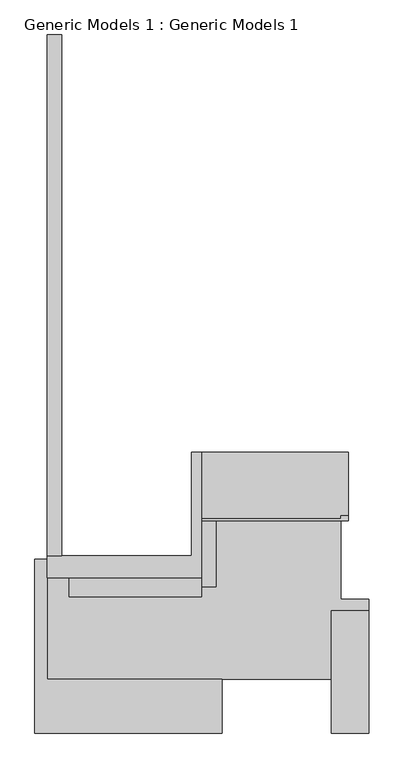
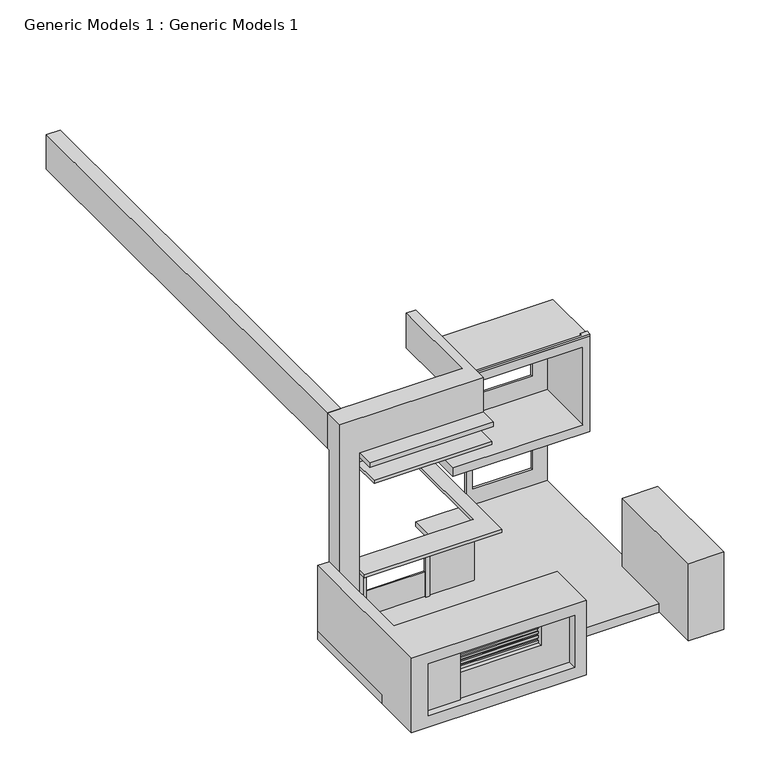
"""IFC4 building model written with IfcOpenShell, lengths in millimetres: proxy geometry, Generic Models 1 : Generic Models 1."""

from ifc_helpers import new_model, si_unit, frame, origin, place, context, project, spatial, polyline, outline, extrude, faceted_brep, source, transform, mapped, element, save


def generic_models_1_generic_models_1_aa7367fc(model_context):
    return source(origin(), model_context, "Body", "SolidModel", [
        extrude(outline(polyline([(-18721.6590927, -15995.5795999), (-19915.2161422, -15995.5795999), (-19915.2161422, -15919.3795999), (-18721.6590927, -15919.3795999), (-18721.6590927, -15995.5795999)])), frame((0.0, 0.0, 243.5207703), z_axis=(0.0, 0.0, 1.0), x_axis=(1.0, 0.0, 0.0)), (0.0, 0.0, 1.0), 1828.8),
        faceted_brep([(-20093.0161422, -14542.885934, 2459.7933128), (-20093.0161422, -10818.9867758, 2459.7933128), (-20474.0161422, -10818.9867758, 2459.7933128), (-20474.0161422, -16224.1795999, 2459.7933128), (-14644.7161422, -16224.1795999, 2459.7933128), (-14644.7161422, -14542.885934, 2459.7933128), (-20474.0161422, -14542.885934, 152.4), (-20474.0161422, -10818.9867758, 152.4), (-20093.0161422, -10818.9867758, 152.4), (-20093.0161422, -14542.885934, 152.4), (-20474.0161422, -14542.885934, -152.4), (-20474.0161422, -16224.1795999, -152.4), (-14644.7161422, -16224.1795999, -152.4), (-15038.4161422, -16224.1795999, 2072.3207703), (-15038.4161422, -16224.1795999, 243.5207703), (-19915.2161422, -16224.1795999, 243.5207703), (-19915.2161422, -16224.1795999, 2072.3207703), (-14644.7161422, -14542.885934, -152.4), (-19915.2161422, -15919.3795999, 2072.3207703), (-19915.2161422, -15919.3795999, 243.5207703), (-15038.4161422, -15919.3795999, 243.5207703), (-15038.4161422, -15919.3795999, 2072.3207703), (-15978.4590927, -15919.3795999, 2072.3207703), (-15978.4590927, -15919.3795999, 1157.9207703), (-18721.6590927, -15919.3795999, 1157.9207703), (-18721.6590927, -15919.3795999, 2072.3207703), (-18721.6590927, -15766.9795999, 2072.3207703), (-15978.4590927, -15766.9795999, 2072.3207703), (-18721.6590927, -15766.9795999, 1981.5649803), (-15978.4590927, -15766.9795999, 1981.5649803), (-18721.6590927, -15766.9795999, 1157.9207703), (-15978.4590927, -15766.9795999, 1157.9207703), (-15978.4590927, -15766.9795999, 1255.1713252), (-18721.6590927, -15766.9795999, 1255.1713252), (-18721.6590927, -15766.9795999, 1838.3053525), (-18721.6590927, -15766.9795999, 1778.0550652), (-15978.4590927, -15766.9795999, 1778.0550652), (-15978.4590927, -15766.9795999, 1838.3053525), (-18721.6590927, -15766.9795999, 1718.5907977), (-18721.6590927, -15766.9795999, 1668.7672478), (-15978.4590927, -15766.9795999, 1668.7672478), (-15978.4590927, -15766.9795999, 1718.5907977), (-18721.6590927, -15766.9795999, 1558.4809342), (-18721.6590927, -15766.9795999, 1493.486018), (-15978.4590927, -15766.9795999, 1493.486018), (-15978.4590927, -15766.9795999, 1558.4809342), (-18721.6590927, -15766.9795999, 1415.4921185), (-18721.6590927, -15766.9795999, 1328.8322303), (-15978.4590927, -15766.9795999, 1328.8322303), (-15978.4590927, -15766.9795999, 1415.4921185), (-15978.4590927, -15716.1795999, 1981.5649803), (-15978.4590927, -15716.1795999, 1838.3053525), (-15978.4590927, -15716.1795999, 1778.0550652), (-15978.4590927, -15716.1795999, 1718.5907977), (-15978.4590927, -15716.1795999, 1668.7672478), (-15978.4590927, -15716.1795999, 1558.4809342), (-15978.4590927, -15716.1795999, 1493.486018), (-15978.4590927, -15716.1795999, 1415.4921185), (-15978.4590927, -15716.1795999, 1328.8322303), (-15978.4590927, -15716.1795999, 1255.1713252), (-18721.6590927, -15716.1795999, 1255.1713252), (-18721.6590927, -15716.1795999, 1328.8322303), (-18721.6590927, -15716.1795999, 1415.4921185), (-18721.6590927, -15716.1795999, 1493.486018), (-18721.6590927, -15716.1795999, 1558.4809342), (-18721.6590927, -15716.1795999, 1668.7672478), (-18721.6590927, -15716.1795999, 1718.5907977), (-18721.6590927, -15716.1795999, 1778.0550652), (-18721.6590927, -15716.1795999, 1838.3053525), (-18721.6590927, -15716.1795999, 1981.5649803)], [[[0, 1, 2, 3, 4, 5]], [[6, 7, 8, 9]], [[1, 0, 9, 8]], [[2, 1, 8, 7]], [[7, 6, 10, 11, 3, 2]], [[12, 4, 3, 11], [13, 14, 15, 16]], [[17, 10, 6, 9, 0, 5]], [[4, 12, 17, 5]], [[12, 11, 10, 17]], [[18, 19, 20, 21, 22, 23, 24, 25]], [[21, 20, 14, 13]], [[20, 19, 15, 14]], [[19, 18, 16, 15]], [[21, 13, 16, 18, 25, 26, 27, 22]], [[27, 26, 28, 29]], [[30, 31, 32, 33]], [[34, 35, 36, 37]], [[38, 39, 40, 41]], [[42, 43, 44, 45]], [[46, 47, 48, 49]], [[31, 23, 22, 27, 29, 50, 51, 37, 36, 52, 53, 41, 40, 54, 55, 45, 44, 56, 57, 49, 48, 58, 59, 32]], [[31, 30, 24, 23]], [[24, 30, 33, 60, 61, 47, 46, 62, 63, 43, 42, 64, 65, 39, 38, 66, 67, 35, 34, 68, 69, 28, 26, 25]], [[50, 69, 68, 51]], [[52, 67, 66, 53]], [[54, 65, 64, 55]], [[56, 63, 62, 57]], [[58, 61, 60, 59]], [[51, 68, 34, 37]], [[69, 50, 29, 28]], [[53, 66, 38, 41]], [[67, 52, 36, 35]], [[55, 64, 42, 45]], [[65, 54, 40, 39]], [[57, 62, 46, 49]], [[63, 56, 44, 43]], [[59, 60, 33, 32]], [[61, 58, 48, 47]]]),
        extrude(outline(polyline([(-10072.7161422, -16224.1795999), (-11248.8984734, -16224.1795999), (-11248.8984734, -12419.1867758), (-10072.7161422, -12419.1867758), (-10072.7161422, -16224.1795999)])), frame((0.0, 0.0, -152.4), z_axis=(0.0, 0.0, 1.0), x_axis=(1.0, 0.0, 0.0)), (0.0, 0.0, 1.0), 2716.6580235),
        faceted_brep([(-19413.0681274, -10971.3867758, 2163.0020846), (-19413.0681274, -10971.3867758, 152.4), (-19038.9161422, -10971.3867758, 152.4), (-19038.9161422, -10971.3867758, 2163.0020846), (-19413.0681274, -10920.5867758, 2163.0020846), (-19038.9161422, -10920.5867758, 2163.0020846), (-19038.9161422, -10920.5867758, 152.4), (-19413.0681274, -10920.5867758, 152.4), (-18911.9161422, -10920.5867758, 2163.0020846), (-18911.9161422, -10920.5867758, 152.4), (-19038.9161422, -10818.9867758, 152.4), (-19038.9161422, -10818.9867758, 2163.0020846), (-18911.9161422, -10818.9867758, 2163.0020846), (-18911.9161422, -10818.9867758, 1025.0994511), (-16930.7161422, -10818.9867758, 1025.0994511), (-16930.7161422, -10818.9867758, 152.4), (-16930.7161422, -10869.7867758, 152.4), (-18911.9161422, -10869.7867758, 152.4), (-18911.9161422, -10869.7867758, 1025.0994511), (-16930.7161422, -10869.7867758, 1025.0994511)], [[[0, 1, 2, 3]], [[4, 5, 6, 7]], [[1, 0, 4, 7]], [[2, 1, 7, 6]], [[3, 2, 6, 5]], [[0, 3, 5, 4]], [[8, 5, 6, 9]], [[10, 11, 12, 13, 14, 15]], [[5, 8, 12, 11]], [[11, 10, 6, 5]], [[9, 6, 10, 15, 16, 17]], [[8, 9, 17, 18, 13, 12]], [[19, 18, 17, 16]], [[18, 19, 14, 13]], [[19, 16, 15, 14]]]),
        extrude(outline(polyline([(-15292.4161422, -10869.7867758), (-16802.5911072, -10869.7867758), (-16802.5911072, -10818.9867758), (-15292.4161422, -10818.9867758), (-15292.4161422, -10869.7867758)])), frame((0.0, 0.0, 152.4), z_axis=(0.0, 0.0, 1.0), x_axis=(1.0, 0.0, 0.0)), (0.0, 0.0, 1.0), 2010.6020846),
        extrude(outline(polyline([(-19219.0295013, -10869.7867758), (-19413.0681274, -10869.7867758), (-19413.0681274, -10818.9867758), (-19219.0295013, -10818.9867758), (-19219.0295013, -10869.7867758)])), frame((0.0, 0.0, 3352.8), z_axis=(0.0, 0.0, 1.0), x_axis=(1.0, 0.0, 0.0)), (0.0, 0.0, 1.0), 2310.6651167),
        extrude(outline(polyline([(-15292.4161422, -10869.7867758), (-19413.0681274, -10869.7867758), (-19413.0681274, -10818.9867758), (-15292.4161422, -10818.9867758), (-15292.4161422, -10869.7867758)])), frame((0.0, 0.0, 5663.4651167), z_axis=(0.0, 0.0, 1.0), x_axis=(1.0, 0.0, 0.0)), (0.0, 0.0, 1.0), 580.3392162),
        extrude(outline(polyline([(-16802.5911072, -10920.5867758), (-16930.7161422, -10920.5867758), (-16930.7161422, -10818.9867758), (-16802.5911072, -10818.9867758), (-16802.5911072, -10920.5867758)])), frame((0.0, 0.0, 152.4), z_axis=(0.0, 0.0, 1.0), x_axis=(1.0, 0.0, 0.0)), (0.0, 0.0, 1.0), 2010.6020846),
        extrude(outline(polyline([(2217.8846358, -10944.2876245), (3048.0, -10944.2876245), (3048.0, -13650.3561315), (152.4, -13650.3561315), (152.4, -10949.0161422), (2217.8846358, -10949.0161422), (2217.8846358, -10944.2876245)]), holes=[polyline([(2217.8846358, -11444.3161422), (714.2961729, -11444.3161422), (714.2961729, -13425.5161422), (2217.8846358, -13425.5161422), (2217.8846358, -11444.3161422)])]), frame((0.0, -7567.7867758, 0.0), z_axis=(0.0, 1.0, 0.0), x_axis=(0.0, 0.0, 1.0)), (0.0, 0.0, 1.0), 76.2),
        extrude(outline(polyline([(-19635.8161422, -10704.6867758), (-20093.0161422, -10704.6867758), (-20093.0161422, 5487.8132242), (-19635.8161422, 5487.8132242), (-19635.8161422, -10704.6867758)])), frame((0.0, 0.0, 6400.8), z_axis=(0.0, 0.0, 1.0), x_axis=(1.0, 0.0, 0.0)), (0.0, 0.0, 1.0), 1219.2),
        extrude(outline(polyline([(6096.0, -13658.1564563), (3352.8, -13658.1564563), (3352.8, -13425.5161422), (3355.4784757, -13425.5161422), (3355.4784757, -10949.0161422), (6096.0, -10949.0161422), (6096.0, -13658.1564563)]), holes=[polyline([(5431.5526731, -11457.0161422), (3998.6028627, -11457.0161422), (3998.6028627, -13425.5161422), (5431.5526731, -13425.5161422), (5431.5526731, -11457.0161422)])]), frame((0.0, -7567.7867758, 0.0), z_axis=(0.0, 1.0, 0.0), x_axis=(0.0, 0.0, 1.0)), (0.0, 0.0, 1.0), 76.2),
        extrude(outline(polyline([(-10720.4161422, -9625.1422165), (-15292.4161422, -9625.1422165), (-15292.4161422, -9563.1336072), (-10949.0161422, -9563.1336072), (-10949.0161422, -9466.2958238), (-10720.4161422, -9466.2958238), (-10720.4161422, -9625.1422165)])), frame((0.0, 0.0, 6400.8), z_axis=(0.0, 0.0, 1.0), x_axis=(1.0, 0.0, 0.0)), (0.0, 0.0, 1.0), 76.2),
        extrude(outline(polyline([(-19413.0681274, -11671.4830509), (-19413.0681274, -10818.9867758), (-15292.4161422, -10818.9867758), (-15292.4161422, -7516.9867758), (-14829.7614132, -7516.9867758), (-14829.7614132, -11671.4830509), (-19413.0681274, -11671.4830509)])), frame((0.0, 0.0, 2163.0020846), z_axis=(0.0, 0.0, 1.0), x_axis=(1.0, 0.0, 0.0)), (0.0, 0.0, 1.0), 101.6),
        extrude(outline(polyline([(-15292.4161422, -10818.9867758), (-15292.4161422, -11897.0390885), (-19216.7161422, -11897.0390885), (-19216.7161422, -10818.9867758), (-15292.4161422, -10818.9867758)])), frame((0.0, 0.0, 5554.6402073), z_axis=(0.0, 0.0, 1.0), x_axis=(1.0, 0.0, 0.0)), (0.0, 0.0, 1.0), 105.6615052),
        extrude(outline(polyline([(-15292.4161422, -11984.5426097), (-19413.0681274, -11984.5426097), (-19413.0681274, -10818.9867758), (-15292.4161422, -10818.9867758), (-15292.4161422, -11984.5426097)])), frame((0.0, 0.0, 6243.8043329), z_axis=(0.0, 0.0, 1.0), x_axis=(1.0, 0.0, 0.0)), (0.0, 0.0, 1.0), 156.9956671),
        faceted_brep([(-20093.0161422, -11395.0766858, 152.4), (-20093.0161422, -11395.0766858, 7620.0), (-20093.0161422, -10704.6867758, 7620.0), (-20093.0161422, -10704.6867758, 6400.8), (-20093.0161422, -10818.9867758, 6400.8), (-20093.0161422, -10818.9867758, 152.4), (-19413.0681274, -11395.0766858, 152.4), (-19413.0681274, -10818.9867758, 152.4), (-19413.0681274, -11395.0766858, 6400.8), (-19413.0681274, -10818.9867758, 6400.8), (-15597.2161422, -7491.5867758, 7620.0), (-15292.4161422, -7491.5867758, 7620.0), (-15292.4161422, -7491.5867758, 6400.8), (-15597.2161422, -7491.5867758, 6400.8), (-15597.2161422, -10704.6867758, 6400.8), (-15597.2161422, -10704.6867758, 7620.0), (-15292.4161422, -11395.0766858, 6400.8), (-15292.4161422, -11395.0766858, 7620.0)], [[[0, 1, 2, 3, 4, 5]], [[6, 0, 5, 7]], [[8, 6, 7, 9]], [[10, 11, 12, 13]], [[10, 13, 14, 15]], [[0, 6, 8, 16, 17, 1]], [[9, 7, 5, 4]], [[1, 17, 11, 10, 15, 2]], [[13, 12, 16, 8, 9, 4, 3, 14]], [[11, 17, 16, 12]], [[2, 15, 14, 3]]]),
        faceted_brep([(-10072.7161422, -12067.3066431, 152.4), (-10072.7161422, -12067.3066431, -152.4), (-15292.4161422, -12067.3066431, -152.4), (-15292.4161422, -12067.3066431, 0.0), (-10949.0161422, -12067.3066431, 0.0), (-10949.0161422, -12067.3066431, 152.4), (-10072.7161422, -14542.885934, -152.4), (-10072.7161422, -14542.885934, 152.4), (-20474.0161422, -14542.885934, -152.4), (-20474.0161422, -14542.885934, 152.4), (-20474.0161422, -10818.9867758, -152.4), (-15292.4161422, -10818.9867758, -152.4), (-20474.0161422, -10818.9867758, 152.4), (-15292.4161422, -10818.9867758, 152.4), (-15292.4161422, -10818.9867758, 0.0), (-15292.4161422, -7491.5867758, 0.0), (-10949.0161422, -7491.5867758, 0.0), (-15292.4161422, -7491.5867758, 152.4), (-10949.0161422, -7491.5867758, 152.4)], [[[0, 1, 2, 3, 4, 5]], [[6, 1, 0, 7]], [[8, 6, 7, 9]], [[10, 11, 2, 1, 6, 8]], [[12, 13, 14, 11, 10]], [[9, 12, 10, 8]], [[11, 14, 3, 2]], [[15, 16, 4, 3, 14]], [[17, 18, 16, 15]], [[17, 15, 14, 13]], [[16, 18, 5, 4]], [[13, 12, 9, 7, 0, 5, 18, 17]]]),
        extrude(outline(polyline([(6400.8, -10720.4161422), (6400.8, -15292.4161422), (6096.0, -15292.4161422), (6096.0, -10949.0161422), (3352.8, -10949.0161422), (3352.8, -15292.4161422), (3048.0, -15292.4161422), (3048.0, -10720.4161422), (6400.8, -10720.4161422)])), frame((0.0, -9625.1422165, 0.0), z_axis=(0.0, 1.0, 0.0), x_axis=(0.0, 0.0, 1.0)), (0.0, 0.0, 1.0), 2133.5554407),
    ])


if __name__ == "__main__":
    model = new_model("IFC4")
    model_context = context("Model", 3, world=origin())
    ifc_project = project(units=[si_unit("LENGTHUNIT", "METRE", prefix="MILLI")], contexts=[model_context])
    site = spatial("IfcSite", under=ifc_project)
    building = spatial("IfcBuilding", under=site)
    placement = place(None, origin())
    generic_models_1_generic_models_1_shape = generic_models_1_generic_models_1_aa7367fc(model_context)
    element("IfcBuildingElementProxy", 1, Name="Generic Models 1 : Generic Models 1", ObjectType="Generic Models 1 : Generic Models 1", at=placement, inside=building, context=model_context, shape_type="MappedRepresentation", body=[
        mapped(generic_models_1_generic_models_1_shape, transform((0.0, 0.0, 0.0), x_axis=(1.0, 0.0, 0.0), y_axis=(0.0, 1.0, 0.0), z_axis=(0.0, 0.0, 1.0))),
    ])
    save(model, "model.ifc")
